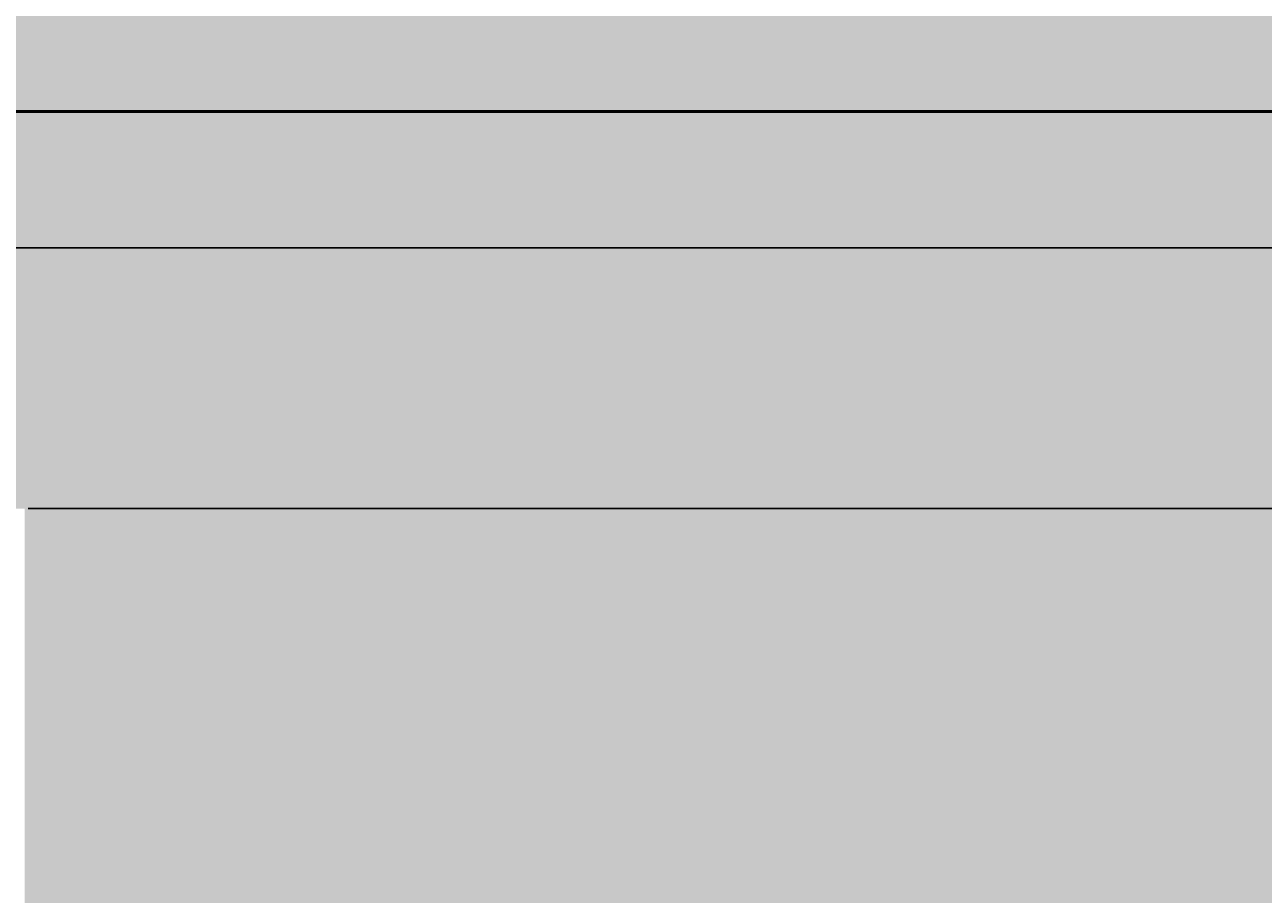
# Model space of a CAD drawing. Units: inches. Extents: x -12 to 334, y -10 to 186.
# Tile 35 of 77: x 106 to 129, y 49 to 65. Entities that reach past the tile are written whole.
import ezdxf

# ---------------------------------------------------------------- set-up
doc = ezdxf.new("R2010")
doc.units = ezdxf.units.IN
doc.header["$MEASUREMENT"] = 0
for name, color, linetype, lineweight in [('M-DIMS', 2, 'Continuous', 18), ('M-EQPM', 7, 'Continuous', 50), ('M-EQPM-PATT', 8, 'Continuous', 18)]:
    doc.layers.add(name, color=color, linetype=linetype, lineweight=lineweight)
doc.styles.get("Standard").update_dxf_attribs({"font": 'arial.ttf'})
doc.dimstyles.get("Standard").update_dxf_attribs({"dimtxt": 0.18, "dimasz": 0.18, "dimexe": 0.18, "dimexo": 0.0625, "dimgap": 0.09, "dimtad": 0, "dimtih": 1, "dimtoh": 1, "dimdec": 4, "dimzin": 0, "dimdsep": 46, "dimtxsty": 'Standard', "dimcen": 0.09, "dimadec": 0, "dimazin": 0, "dimtfac": 1, "dimtdec": 4, "dimtofl": 0, "dimtmove": 0, "dimatfit": 3, "dimfxl": 1, "dimtolj": 1, "dimtzin": 0, "dimarcsym": 0})

# ---------------------------------------------------------------- blocks, each defined once
blk = doc.blocks.new('*D1')
at = {"layer": 'Defpoints', "color": 0, "transparency": 16777216}
for p in [(281.426, 91.899), (3.376, 80.692), (281.426, 14.304)]:
    blk.add_point(p, dxfattribs=at)
at = {"layer": 'M-DIMS', "color": 0, "lineweight": -2, "transparency": 16777216}
for p, q in [((281.426, 91.836), (281.426, 14.124)), ((3.376, 80.629), (3.376, 14.124)), ((3.556, 14.304), (141.935, 14.304)), ((281.246, 14.304), (142.867, 14.304))]:
    blk.add_line(p, q, dxfattribs=at)
at = {"layer": 'M-DIMS', "color": 0, "transparency": 16777216}
for points in [[(3.556, 14.334), (3.556, 14.274), (3.376, 14.304)], [(281.246, 14.334), (281.246, 14.274), (281.426, 14.304)]]:
    blk.add_solid(points, dxfattribs=at)
at = {"layer": 'M-DIMS', "color": 0, "transparency": 16777216, "insert": (142.401, 14.304), "char_height": 0.18, "attachment_point": 5}
blk.add_mtext('\\A1;278.05', dxfattribs=at)
blk = doc.blocks.new('*D17')
at = {"layer": 'Defpoints', "color": 0, "transparency": 16777216}
for p in [(106.177, 102.896), (105.892, 56.321), (295.976, 56.321)]:
    blk.add_point(p, dxfattribs=at)
at = {"layer": 'M-DIMS', "color": 0, "lineweight": -2, "transparency": 16777216}
for p, q in [((106.24, 102.896), (296.156, 102.896)), ((295.976, 102.716), (295.976, 79.79)), ((295.976, 56.501), (295.976, 79.426)), ((105.954, 56.321), (296.156, 56.321))]:
    blk.add_line(p, q, dxfattribs=at)
at = {"layer": 'M-DIMS', "color": 0, "transparency": 16777216}
for points in [[(295.946, 102.716), (296.006, 102.716), (295.976, 102.896)], [(295.946, 56.501), (296.006, 56.501), (295.976, 56.321)]]:
    blk.add_solid(points, dxfattribs=at)
at = {"layer": 'M-DIMS', "color": 0, "transparency": 16777216, "insert": (295.976, 79.608), "char_height": 0.18, "attachment_point": 5}
blk.add_mtext('\\A1;46.575', dxfattribs=at)
blk = doc.blocks.new('*D30')
at = {"layer": 'Defpoints', "color": 0, "transparency": 16777216}
for p in [(75.924, 63.612), (129.093, 61.105), (129.093, 14.304)]:
    blk.add_point(p, dxfattribs=at)
at = {"layer": 'M-DIMS', "color": 0, "lineweight": -2, "transparency": 16777216}
for p, q in [((75.924, 63.549), (75.924, 14.124)), ((129.093, 61.042), (129.093, 14.124)), ((76.104, 14.304), (102.115, 14.304)), ((128.913, 14.304), (102.902, 14.304))]:
    blk.add_line(p, q, dxfattribs=at)
at = {"layer": 'M-DIMS', "color": 0, "transparency": 16777216}
for points in [[(76.104, 14.334), (76.104, 14.274), (75.924, 14.304)], [(128.913, 14.334), (128.913, 14.274), (129.093, 14.304)]]:
    blk.add_solid(points, dxfattribs=at)
at = {"layer": 'M-DIMS', "color": 0, "transparency": 16777216, "insert": (102.509, 14.304), "char_height": 0.18, "attachment_point": 5}
blk.add_mtext('\\A1;53.17', dxfattribs=at)
blk = doc.blocks.new('*D35')
at = {"layer": 'Defpoints', "color": 0, "transparency": 16777216}
for p in [(216.428, 98.108), (-11.174, 61.105), (216.428, 61.105)]:
    blk.add_point(p, dxfattribs=at)
at = {"layer": 'M-DIMS', "color": 0, "lineweight": -2, "transparency": 16777216}
for p, q in [((216.365, 98.108), (-11.354, 98.108)), ((-11.174, 97.928), (-11.174, 79.788)), ((-11.174, 61.285), (-11.174, 79.424)), ((216.365, 61.105), (-11.354, 61.105))]:
    blk.add_line(p, q, dxfattribs=at)
at = {"layer": 'M-DIMS', "color": 0, "transparency": 16777216}
for points in [[(-11.204, 97.928), (-11.144, 97.928), (-11.174, 98.108)], [(-11.204, 61.285), (-11.144, 61.285), (-11.174, 61.105)]]:
    blk.add_solid(points, dxfattribs=at)
at = {"layer": 'M-DIMS', "color": 0, "transparency": 16777216, "insert": (-11.174, 79.606), "char_height": 0.18, "attachment_point": 5}
blk.add_mtext('\\A1;37', dxfattribs=at)
blk = doc.blocks.new('*D39')
at = {"layer": 'Defpoints', "color": 0, "transparency": 16777216}
for p in [(279.726, 80.692), (-11.174, 45.854), (269.381, 45.854)]:
    blk.add_point(p, dxfattribs=at)
at = {"layer": 'M-DIMS', "color": 0, "lineweight": -2, "transparency": 16777216}
for p, q in [((279.664, 80.692), (-11.354, 80.692)), ((-11.174, 80.512), (-11.174, 63.455)), ((-11.174, 46.034), (-11.174, 63.091)), ((269.318, 45.854), (-11.354, 45.854))]:
    blk.add_line(p, q, dxfattribs=at)
at = {"layer": 'M-DIMS', "color": 0, "transparency": 16777216}
for points in [[(-11.204, 80.512), (-11.144, 80.512), (-11.174, 80.692)], [(-11.204, 46.034), (-11.144, 46.034), (-11.174, 45.854)]]:
    blk.add_solid(points, dxfattribs=at)
at = {"layer": 'M-DIMS', "color": 0, "transparency": 16777216, "insert": (-11.174, 63.273), "char_height": 0.18, "attachment_point": 5}
blk.add_mtext('\\A1;34.84', dxfattribs=at)

msp = doc.modelspace()

# ---------------------------------------------------------------- hatches: boundary and pattern name
at = {"layer": 'M-EQPM-PATT'}
h = msp.add_hatch(color=256, dxfattribs=at)
h.set_gradient(color1=(205, 32, 39), color2=(205, 32, 39), tint=1)
h.paths.add_polyline_path([(64.5, 80.754), (64.5, 89.8963), (226.6083, 89.8963, -1), (226.6083, 69.6117), (64.5, 69.6117), (64.5, 78.754), (4.4744, 78.754, 0.384914), (23.5807, 61.4872), (37.1002, 61.4872), (37.1002, 33.6752), (53.1002, 33.6752), (53.1002, 61.4872), (64.5, 61.4872), (64.5, 63.6117), (226.6083, 63.6117, 1), (226.6083, 95.8963), (64.5, 95.8963), (64.5, 99.8958), (53.1002, 99.8958), (53.1002, 127.7078), (37.1002, 127.7078), (37.1002, 99.8958), (23.5807, 99.8958, 0.4132606), (4.3766, 80.754)])
h.paths.add_polyline_path([(64.5, 91.8963), (64.5, 93.8963), (226.6083, 93.8963, -1), (226.6083, 65.6117), (64.5, 65.6117), (64.5, 67.6117), (226.6083, 67.6117, 1), (226.6083, 91.8963)], flags=16)
h = msp.add_hatch(color=256, dxfattribs=at)
h.set_gradient(color1=(94, 103, 175), color2=(94, 103, 175), tint=1)
h.paths.add_polyline_path([(129.093, 89.8963), (86.8879, 89.8963), (86.8879, 69.6117), (129.093, 69.6117)], flags=17)
h.paths.add_polyline_path([(170.9079, 89.8963), (130.8573, 89.8963), (130.8573, 69.6117), (170.9079, 69.6117)], flags=17)
h.paths.add_polyline_path([(216.4278, 89.8963), (172.6722, 89.8963), (172.6722, 69.6117), (216.4278, 69.6117)], flags=17)
h.paths.add_polyline_path([(245.9354, 82.6969), (247.9354, 82.6969), (247.9354, 46.8541), (268.3808, 46.8541, 0.0998398), (279.7263, 80.6915), (251.9801, 80.6915, 0.4142136), (231.7758, 100.8958), (84.7229, 100.8958), (84.7229, 109.0583), (83.7229, 109.0583), (83.7229, 95.8963), (129.093, 95.8963), (129.093, 98.1081), (130.8573, 98.1081), (130.8573, 95.8963), (170.9079, 95.8963), (170.9079, 98.1081), (172.6722, 98.1081), (172.6722, 95.8963), (216.4278, 95.8963), (216.4278, 98.1081), (218.1922, 98.1081), (218.1922, 95.8963), (226.6083, 95.8963, -1), (226.6083, 63.6117), (218.1922, 63.6117), (218.1922, 61.1045), (216.4278, 61.1045), (216.4278, 63.6117), (172.6722, 63.6117), (172.6722, 61.1045), (170.9079, 61.1045), (170.9079, 63.6117), (130.8573, 63.6117), (130.8573, 61.1045), (129.093, 61.1045), (129.093, 63.6117), (87.8879, 63.6117), (87.8879, 56.3205), (105.8919, 56.3205), (105.8919, 28.8541), (115.8919, 28.8541), (115.8919, 46.8541), (222.5761, 46.8541), (222.5761, 30.8541), (232.5761, 30.8541), (232.5761, 46.8541), (245.9354, 46.8541)])
h.paths.add_polyline_path([(86.8879, 89.8963), (75.9244, 89.8963), (75.9244, 69.6117), (86.8879, 69.6117)])
h.paths.add_polyline_path([(83.7229, 109.0583), (75.9244, 109.0583), (75.9244, 95.8963), (83.7229, 95.8963)])
h.paths.add_polyline_path([(226.6083, 89.8963), (218.1922, 89.8963), (218.1922, 69.6117), (226.6083, 69.6117, 1)], flags=17)
h = msp.add_hatch(color=256, dxfattribs=at)
h.set_gradient(color1=(0, 0, 255), color2=(0, 0, 255), tint=1)
h.paths.add_polyline_path([(84.7229, 100.8958), (84.7229, 109.0583), (83.7229, 109.0583), (83.7229, 95.8963), (129.093, 95.8963), (129.093, 98.1081), (130.8573, 98.1081), (130.8573, 95.8963), (170.9079, 95.8963), (170.9079, 98.1081), (172.6722, 98.1081), (172.6722, 95.8963), (216.4278, 95.8963), (216.4278, 98.1081), (218.1922, 98.1081), (218.1922, 95.8963), (226.6083, 95.8963, -1), (226.6083, 63.6117), (218.1922, 63.6117), (218.1922, 61.1045), (216.4278, 61.1045), (216.4278, 63.6117), (172.6722, 63.6117), (172.6722, 61.1045), (170.9079, 61.1045), (170.9079, 63.6117), (130.8573, 63.6117), (130.8573, 61.1045), (129.093, 61.1045), (129.093, 63.6117), (87.8879, 63.6117), (87.8879, 56.3205), (105.8919, 56.3205), (105.8919, 28.8541), (115.8919, 28.8541), (115.8919, 46.8541), (222.5761, 46.8541), (222.5761, 30.8541), (232.5761, 30.8541), (232.5761, 46.8541), (245.9354, 46.8541), (245.9354, 82.6969), (247.9354, 82.6969), (247.9354, 46.8541), (268.3808, 46.8541, 0.0998398), (279.7263, 80.6915), (251.9801, 80.6915, 0.4142136), (231.7758, 100.8958)])

# ---------------------------------------------------------------- linework, layer by layer
at = {"layer": 'M-EQPM'}
msp.add_lwpolyline([(64.5, 63.6117), (226.6083, 63.6117, 1), (226.6083, 95.8963), (64.5, 95.8963)], format="xyb", dxfattribs=at)

# ---------------------------------------------------------------- dimensions: what is measured, and where the dimension line sits
at = {"layer": 'M-DIMS'}
for base, p1, p2, override, picture, middle in [((295.9756, 56.3205), (106.1771, 102.8958), (105.8919, 56.3205), {"dimdec": 3, "dimlfac": 1, "dimrnd": 0, "dimzin": 0, "dimdsep": 46, "dimlunit": 2}, '*D17', (295.9756, 79.6082)), ((-11.1736, 61.1045), (216.4278, 98.1081), (216.4278, 61.1045), {"dimdec": 0, "dimlfac": 1, "dimrnd": 0, "dimzin": 0, "dimdsep": 46, "dimlunit": 2}, '*D35', (-11.1735, 79.6063)), ((-11.1736, 45.8541), (279.7263, 80.6915), (269.3808, 45.8541), {"dimdec": 2, "dimlfac": 1, "dimrnd": 0, "dimzin": 0, "dimdsep": 46, "dimlunit": 2}, '*D39', (-11.1735, 63.2728))]:
    dim = msp.add_linear_dim(base=base, p1=p1, p2=p2, angle=90, dimstyle='Standard', override=override, dxfattribs=at)
    dim.commit()
    dim.dimension.update_dxf_attribs({"geometry": picture, "text_midpoint": middle})
for base, p1, p2, picture, middle in [((281.4256, 14.3041), (3.3765, 80.6915), (281.4256, 91.8988), '*D1', (142.401, 14.3041)), ((129.093, 14.3041), (75.9244, 63.6117), (129.093, 61.1045), '*D30', (102.5087, 14.3041))]:
    dim = msp.add_linear_dim(base=base, p1=p1, p2=p2, dimstyle='Standard', override={"dimdec": 2, "dimlfac": 1, "dimrnd": 0, "dimzin": 0, "dimdsep": 46, "dimlunit": 2}, dxfattribs=at)
    dim.commit()
    dim.dimension.update_dxf_attribs({"geometry": picture, "text_midpoint": middle})

doc.saveas('drawing.dxf')
